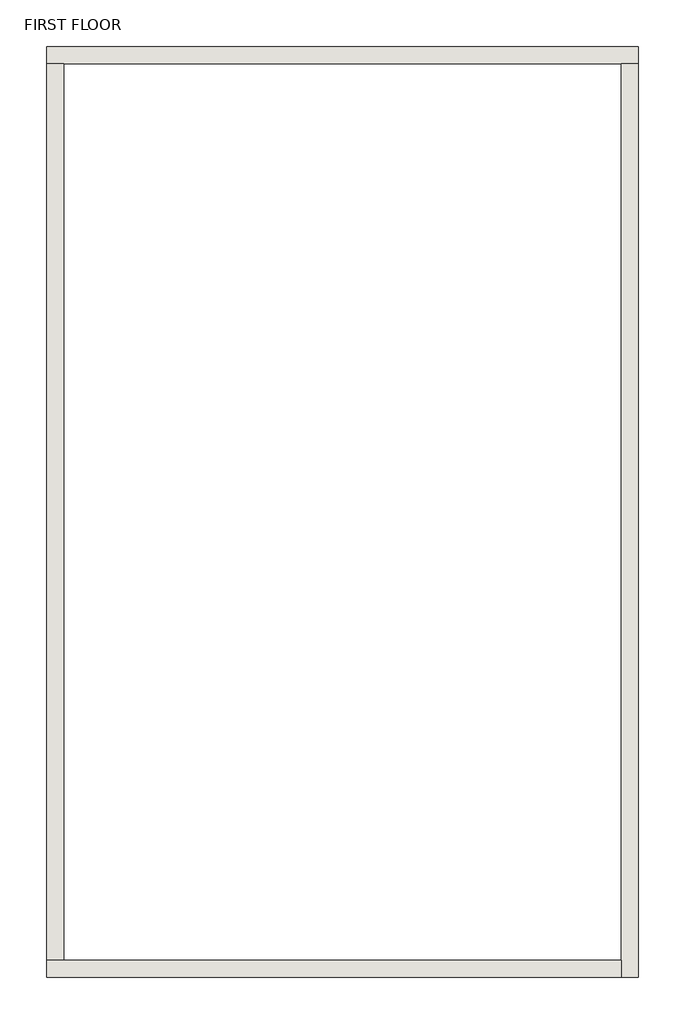
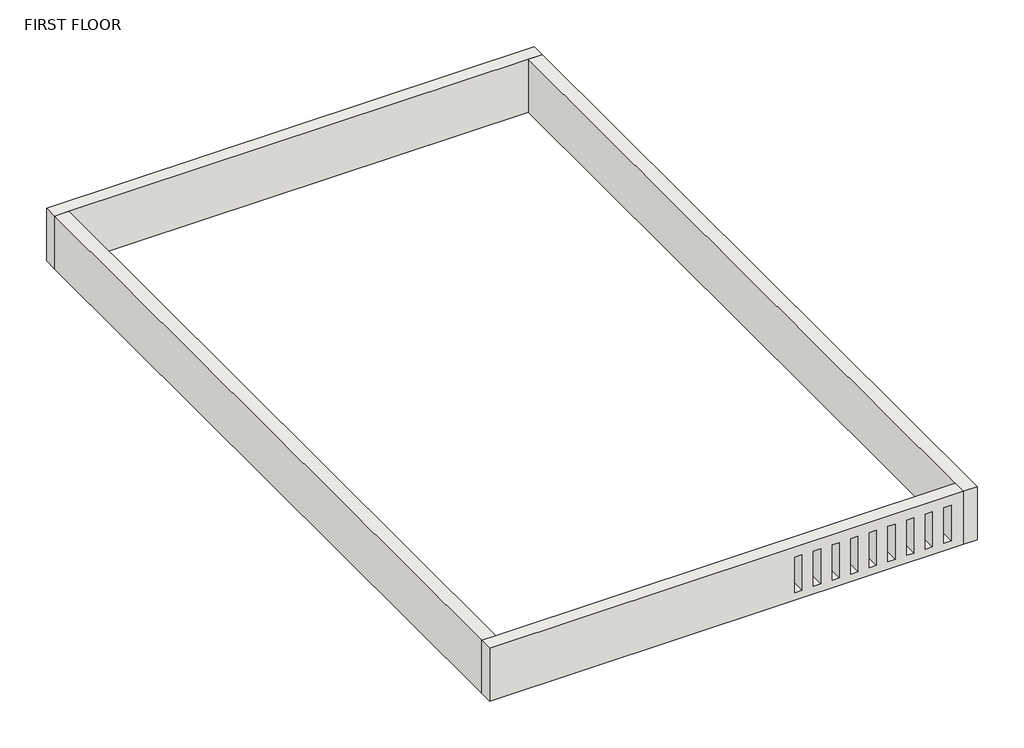
# One storey: 4 walls.
"""IFC4 building model written with IfcOpenShell, lengths in millimetres."""

from ifc_helpers import new_model, si_unit, frame, origin, place, context, project, spatial, polyline, outline, extrude, faceted_brep, element, save

model = new_model("IFC4")

# Units and contexts
model_context = context("Model", 3, world=origin())
ifc_project = project(units=[si_unit("LENGTHUNIT", "METRE", prefix="MILLI")], contexts=[model_context])

# Site, building, storey
site = spatial("IfcSite", under=ifc_project)
building = spatial("IfcBuilding", under=site)
storey = spatial("IfcBuildingStorey", under=building, Name="FIRST FLOOR", Elevation=6096.0)

# Walls
placement = place(None, origin())
element("IfcWall", 1, ObjectType="WALL 9\"", at=placement, inside=storey, context=model_context, shape_type="Brep", body=[
    faceted_brep([(-8482.1519453, 16291.0444012, 6096.0), (-8253.5519453, 16291.0444012, 6096.0), (-735.1519453, 16291.0444012, 6096.0), (-506.5519453, 16291.0444012, 6096.0), (-506.5519453, 16291.0444012, 7010.4), (-735.1519453, 16291.0444012, 7010.4), (-8253.5519453, 16291.0444012, 7010.4), (-8482.1519453, 16291.0444012, 7010.4), (-8482.1519453, 16519.6444012, 6096.0), (-8482.1519453, 16519.6444012, 7010.4), (-506.5519453, 16519.6444012, 7010.4), (-506.5519453, 16519.6444012, 6096.0)], [[[0, 1, 2, 3, 4, 5, 6, 7]], [[8, 9, 10, 11]], [[3, 2, 1, 0, 8, 11]], [[7, 6, 5, 4, 10, 9]], [[4, 3, 11, 10]], [[0, 7, 9, 8]]]),
])
element("IfcWall", 2, ObjectType="WALL 9\"", at=placement, inside=storey, context=model_context, shape_type="Brep", body=[
    faceted_brep([(-735.1519453, 16291.0444012, 6096.0), (-735.1519453, 4200.6444012, 6096.0), (-735.1519453, 3972.0444012, 6096.0), (-735.1519453, 3972.0444012, 7010.4), (-735.1519453, 4200.6444012, 7010.4), (-735.1519453, 16291.0444012, 7010.4), (-506.5519453, 16291.0444012, 6096.0), (-506.5519453, 16291.0444012, 7010.4), (-506.5519453, 3972.0444012, 7010.4), (-506.5519453, 3972.0444012, 6096.0)], [[[0, 1, 2, 3, 4, 5]], [[6, 7, 8, 9]], [[2, 1, 0, 6, 9]], [[5, 4, 3, 8, 7]], [[0, 5, 7, 6]], [[3, 2, 9, 8]]]),
])
element("IfcWall", 3, ObjectType="WALL 9\"", at=placement, inside=storey, context=model_context, shape_type="Brep", body=[
    faceted_brep([(-735.1519453, 4200.6444012, 6096.0), (-8253.5519453, 4200.6444012, 6096.0), (-8482.1519453, 4200.6444012, 6096.0), (-8482.1519453, 4200.6444012, 7010.4), (-8253.5519453, 4200.6444012, 7010.4), (-735.1519453, 4200.6444012, 7010.4), (-3376.7519453, 4200.6444012, 6227.7952096), (-3376.7519453, 4200.6444012, 6837.5860075), (-3493.9691579, 4200.6444012, 6837.5860075), (-3493.9691579, 4200.6444012, 6227.7952096), (-3071.9519453, 4200.6444012, 6227.7952096), (-3071.9519453, 4200.6444012, 6837.5860075), (-3189.1691579, 4200.6444012, 6837.5860075), (-3189.1691579, 4200.6444012, 6227.7952096), (-2767.1519453, 4200.6444012, 6227.7952096), (-2767.1519453, 4200.6444012, 6837.5860075), (-2884.3691579, 4200.6444012, 6837.5860075), (-2884.3691579, 4200.6444012, 6227.7952096), (-2462.3519453, 4200.6444012, 6227.7952096), (-2462.3519453, 4200.6444012, 6837.5860075), (-2579.5691579, 4200.6444012, 6837.5860075), (-2579.5691579, 4200.6444012, 6227.7952096), (-2157.5519453, 4200.6444012, 6227.7952096), (-2157.5519453, 4200.6444012, 6837.5860075), (-2274.7691579, 4200.6444012, 6837.5860075), (-2274.7691579, 4200.6444012, 6227.7952096), (-1852.7519453, 4200.6444012, 6227.7952096), (-1852.7519453, 4200.6444012, 6837.5860075), (-1969.9691579, 4200.6444012, 6837.5860075), (-1969.9691579, 4200.6444012, 6227.7952096), (-1547.9519453, 4200.6444012, 6227.7952096), (-1547.9519453, 4200.6444012, 6837.5860075), (-1665.1691579, 4200.6444012, 6837.5860075), (-1665.1691579, 4200.6444012, 6227.7952096), (-1243.1519453, 4200.6444012, 6227.7952096), (-1243.1519453, 4200.6444012, 6837.5860075), (-1360.3691579, 4200.6444012, 6837.5860075), (-1360.3691579, 4200.6444012, 6227.7952096), (-938.3519453, 4200.6444012, 6227.7952096), (-938.3519453, 4200.6444012, 6837.5860075), (-1055.5691579, 4200.6444012, 6837.5860075), (-1055.5691579, 4200.6444012, 6227.7952096), (-8482.1519453, 3972.0444012, 6096.0), (-735.1519453, 3972.0444012, 6096.0), (-735.1519453, 3972.0444012, 7010.4), (-8482.1519453, 3972.0444012, 7010.4), (-3376.7519453, 3972.0444012, 6837.5860075), (-3376.7519453, 3972.0444012, 6227.7952096), (-3493.9691579, 3972.0444012, 6227.7952096), (-3493.9691579, 3972.0444012, 6837.5860075), (-3071.9519453, 3972.0444012, 6837.5860075), (-3071.9519453, 3972.0444012, 6227.7952096), (-3189.1691579, 3972.0444012, 6227.7952096), (-3189.1691579, 3972.0444012, 6837.5860075), (-2767.1519453, 3972.0444012, 6837.5860075), (-2767.1519453, 3972.0444012, 6227.7952096), (-2884.3691579, 3972.0444012, 6227.7952096), (-2884.3691579, 3972.0444012, 6837.5860075), (-2462.3519453, 3972.0444012, 6837.5860075), (-2462.3519453, 3972.0444012, 6227.7952096), (-2579.5691579, 3972.0444012, 6227.7952096), (-2579.5691579, 3972.0444012, 6837.5860075), (-2157.5519453, 3972.0444012, 6837.5860075), (-2157.5519453, 3972.0444012, 6227.7952096), (-2274.7691579, 3972.0444012, 6227.7952096), (-2274.7691579, 3972.0444012, 6837.5860075), (-1852.7519453, 3972.0444012, 6837.5860075), (-1852.7519453, 3972.0444012, 6227.7952096), (-1969.9691579, 3972.0444012, 6227.7952096), (-1969.9691579, 3972.0444012, 6837.5860075), (-1547.9519453, 3972.0444012, 6837.5860075), (-1547.9519453, 3972.0444012, 6227.7952096), (-1665.1691579, 3972.0444012, 6227.7952096), (-1665.1691579, 3972.0444012, 6837.5860075), (-1243.1519453, 3972.0444012, 6837.5860075), (-1243.1519453, 3972.0444012, 6227.7952096), (-1360.3691579, 3972.0444012, 6227.7952096), (-1360.3691579, 3972.0444012, 6837.5860075), (-938.3519453, 3972.0444012, 6837.5860075), (-938.3519453, 3972.0444012, 6227.7952096), (-1055.5691579, 3972.0444012, 6227.7952096), (-1055.5691579, 3972.0444012, 6837.5860075)], [[[0, 1, 2, 3, 4, 5], [6, 7, 8, 9], [10, 11, 12, 13], [14, 15, 16, 17], [18, 19, 20, 21], [22, 23, 24, 25], [26, 27, 28, 29], [30, 31, 32, 33], [34, 35, 36, 37], [38, 39, 40, 41]], [[42, 43, 44, 45], [46, 47, 48, 49], [50, 51, 52, 53], [54, 55, 56, 57], [58, 59, 60, 61], [62, 63, 64, 65], [66, 67, 68, 69], [70, 71, 72, 73], [74, 75, 76, 77], [78, 79, 80, 81]], [[2, 1, 0, 43, 42]], [[5, 4, 3, 45, 44]], [[0, 5, 44, 43]], [[3, 2, 42, 45]], [[46, 7, 6, 47]], [[47, 6, 9, 48]], [[48, 9, 8, 49]], [[7, 46, 49, 8]], [[50, 11, 10, 51]], [[51, 10, 13, 52]], [[52, 13, 12, 53]], [[11, 50, 53, 12]], [[54, 15, 14, 55]], [[55, 14, 17, 56]], [[56, 17, 16, 57]], [[15, 54, 57, 16]], [[58, 19, 18, 59]], [[59, 18, 21, 60]], [[60, 21, 20, 61]], [[19, 58, 61, 20]], [[62, 23, 22, 63]], [[63, 22, 25, 64]], [[64, 25, 24, 65]], [[23, 62, 65, 24]], [[66, 27, 26, 67]], [[67, 26, 29, 68]], [[68, 29, 28, 69]], [[27, 66, 69, 28]], [[70, 31, 30, 71]], [[71, 30, 33, 72]], [[72, 33, 32, 73]], [[31, 70, 73, 32]], [[74, 35, 34, 75]], [[75, 34, 37, 76]], [[76, 37, 36, 77]], [[35, 74, 77, 36]], [[78, 39, 38, 79]], [[79, 38, 41, 80]], [[80, 41, 40, 81]], [[39, 78, 81, 40]]]),
])
element("IfcWall", 4, ObjectType="WALL 9\"", at=placement, inside=storey, context=model_context, shape_type="SweptSolid", body=[
    extrude(outline(polyline([(-8253.5519453, 16291.0444012), (-8253.5519453, 4200.6444012), (-8482.1519453, 4200.6444012), (-8482.1519453, 16291.0444012), (-8253.5519453, 16291.0444012)])), frame((0.0, 0.0, 6096.0), z_axis=(0.0, 0.0, 1.0), x_axis=(1.0, 0.0, 0.0)), (0.0, 0.0, 1.0), 914.4),
])

save(model, "model.ifc")

# Revit data of these elements
# Type "WALL 9\""
#   Assembly Code = "B2010"
#   Layers, outside or top first: 0' - 9" no material (function 1)
# Elements 1, 2, 3 (IfcWall, "WALL 9\"")
#   Top Offset = 0' - 0"
#   Base Offset = 0' - 0"
#   wall height = 3' - 0"
#   Phase Created = New Construction
#   Base Constraint = FIRST FLOOR
#   Materials on its faces: "Default Wall", "1 wall paint"
# Element 4 (IfcWall, "WALL 9\"")
#   Top Offset = 0' - 0"
#   Base Offset = 0' - 0"
#   wall height = 3' - 0"
#   Phase Created = New Construction
#   Base Constraint = FIRST FLOOR
#   Materials on its faces: "Default Wall"
# Materials
#   "Default Wall": colour RGB 128 128 128, transparency 0, Cost = 0
#   "1 wall paint": class "Generic", colour RGB 120 120 120, transparency 0, Cost = 0
